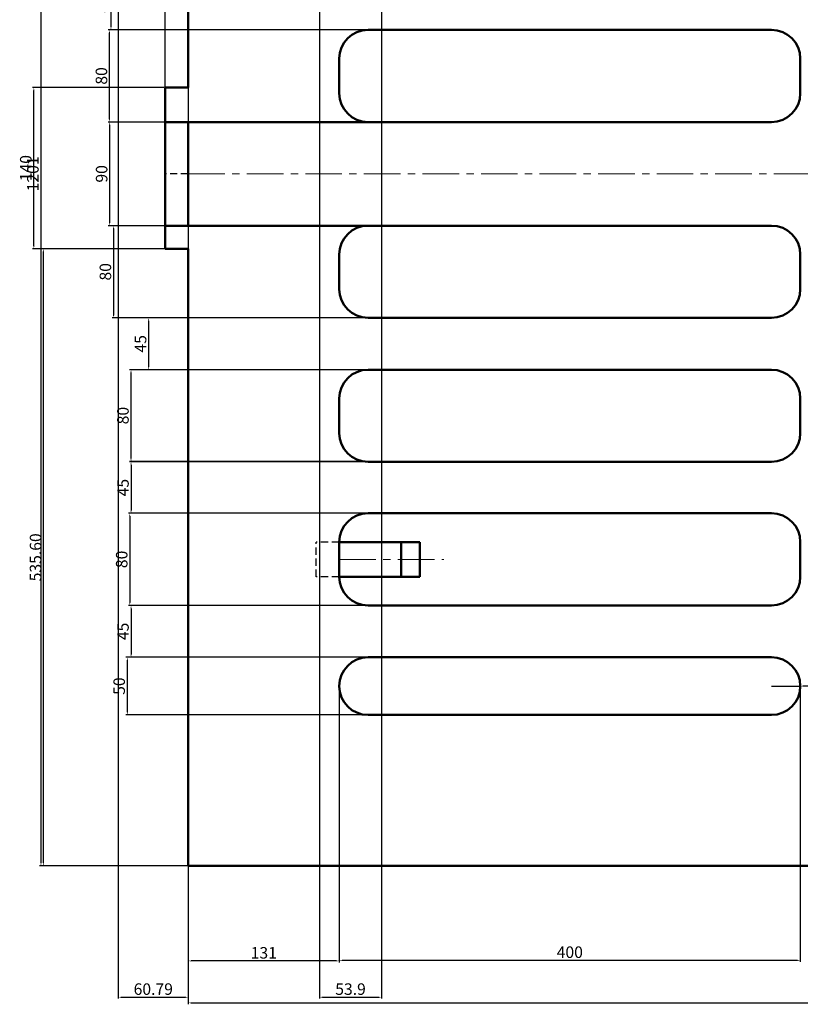
# Model space of a CAD drawing. Units: millimetres. Extents: x 1178 to 3717, y 924 to 2764.
# Tile 2 of 5: x 1793 to 2471, y 931 to 1785. Entities that reach past the tile are written whole.
import ezdxf

# ---------------------------------------------------------------- set-up
doc = ezdxf.new("R2010")
doc.units = ezdxf.units.MM
doc.linetypes.add('CENTER', pattern=[50.8, 31.75, -6.35, 6.35, -6.35])
doc.linetypes.add('HIDDEN', pattern=[9.525, 6.35, -3.175])
for name, color, linetype, lineweight in [('M-CNTR', 1, 'CENTER', 18), ('M-DIMS', 2, 'Continuous', 25), ('M-HIDN', 6, 'HIDDEN', 25), ('M-OUTL', 7, 'Continuous', 50)]:
    doc.layers.add(name, color=color, linetype=linetype, lineweight=lineweight)
doc.styles.get("Standard").update_dxf_attribs({"font": 'arial.ttf'})
doc.dimstyles.new('ISO-25', dxfattribs={"dimtxt": 10, "dimasz": 2.5, "dimexe": 1.25, "dimexo": 0.625, "dimtad": 1, "dimtoh": 1, "dimdec": 0, "dimtxsty": 'Standard', "dimcen": 2.5, "dimadec": 0, "dimazin": 0, "dimtfac": 1, "dimtdec": 0, "dimtmove": 0, "dimatfit": 3, "dimfxl": 1, "dimarcsym": 0})

# ---------------------------------------------------------------- blocks, each defined once
blk = doc.blocks.new('*D1')
at = {"layer": 'Defpoints', "color": 0, "transparency": 16777216}
for p in [(1939.54, 1051.02), (3521.54, 1051.02), (3521.54, 932.11)]:
    blk.add_point(p, dxfattribs=at)
at = {"layer": 'M-DIMS', "color": 0, "lineweight": -2, "transparency": 16777216}
for p, q in [((1939.54, 1050.4), (1939.54, 930.86)), ((3521.54, 1050.4), (3521.54, 930.86)), ((1942.04, 932.11), (3519.04, 932.11))]:
    blk.add_line(p, q, dxfattribs=at)
at = {"layer": 'M-DIMS', "color": 0, "transparency": 16777216}
for points in [[(1942.04, 932.53), (1942.04, 931.7), (1939.54, 932.11)], [(3519.04, 932.53), (3519.04, 931.7), (3521.54, 932.11)]]:
    blk.add_solid(points, dxfattribs=at)
at = {"layer": 'M-DIMS', "color": 0, "transparency": 16777216, "insert": (2730.54, 937.85), "char_height": 10, "attachment_point": 5}
blk.add_mtext('1582', dxfattribs=at)
blk = doc.blocks.new('*D2')
at = {"layer": 'Defpoints', "color": 0, "transparency": 16777216}
for p in [(1939.54, 2252.21), (1811.7, 1051.02), (1939.54, 1051.02)]:
    blk.add_point(p, dxfattribs=at)
at = {"layer": 'M-DIMS', "color": 0, "lineweight": -2, "transparency": 16777216}
for p, q in [((1938.91, 2252.21), (1810.45, 2252.21)), ((1811.7, 2249.71), (1811.7, 1053.52)), ((1938.91, 1051.02), (1810.45, 1051.02))]:
    blk.add_line(p, q, dxfattribs=at)
at = {"layer": 'M-DIMS', "color": 0, "transparency": 16777216}
for points in [[(1811.29, 2249.71), (1812.12, 2249.71), (1811.7, 2252.21)], [(1811.29, 1053.52), (1812.12, 1053.52), (1811.7, 1051.02)]]:
    blk.add_solid(points, dxfattribs=at)
at = {"layer": 'M-DIMS', "color": 0, "transparency": 16777216, "insert": (1805.97, 1651.62), "char_height": 10, "attachment_point": 5, "rotation": 90}
blk.add_mtext('1201', dxfattribs=at)
blk = doc.blocks.new('*D3')
at = {"layer": 'Defpoints', "color": 0, "transparency": 16777216}
for p in [(2070.54, 1207.02), (2470.54, 1207.02), (2470.54, 969.06)]:
    blk.add_point(p, dxfattribs=at)
at = {"layer": 'M-DIMS', "color": 0, "lineweight": -2, "transparency": 16777216}
for p, q in [((2070.54, 1206.4), (2070.54, 967.81)), ((2470.54, 1206.4), (2470.54, 967.81)), ((2073.04, 969.06), (2468.04, 969.06))]:
    blk.add_line(p, q, dxfattribs=at)
at = {"layer": 'M-DIMS', "color": 0, "transparency": 16777216}
for points in [[(2073.04, 969.48), (2073.04, 968.64), (2070.54, 969.06)], [(2468.04, 969.48), (2468.04, 968.64), (2470.54, 969.06)]]:
    blk.add_solid(points, dxfattribs=at)
at = {"layer": 'M-DIMS', "color": 0, "transparency": 16777216, "insert": (2270.54, 974.79), "char_height": 10, "attachment_point": 5}
blk.add_mtext('400', dxfattribs=at)
blk = doc.blocks.new('*D6')
at = {"layer": 'Defpoints', "color": 0, "transparency": 16777216}
for p in [(2095.54, 1232.02), (1886.58, 1182.02), (2095.54, 1182.02)]:
    blk.add_point(p, dxfattribs=at)
at = {"layer": 'M-DIMS', "color": 0, "lineweight": -2, "transparency": 16777216}
for p, q in [((2094.91, 1232.02), (1885.33, 1232.02)), ((1886.58, 1229.52), (1886.58, 1184.52)), ((2094.91, 1182.02), (1885.33, 1182.02))]:
    blk.add_line(p, q, dxfattribs=at)
at = {"layer": 'M-DIMS', "color": 0, "transparency": 16777216}
for points in [[(1886.16, 1229.52), (1886.99, 1229.52), (1886.58, 1232.02)], [(1886.16, 1184.52), (1886.99, 1184.52), (1886.58, 1182.02)]]:
    blk.add_solid(points, dxfattribs=at)
at = {"layer": 'M-DIMS', "color": 0, "transparency": 16777216, "insert": (1880.85, 1207.02), "char_height": 10, "attachment_point": 5, "rotation": 90}
blk.add_mtext('50', dxfattribs=at)
blk = doc.blocks.new('*D7')
at = {"layer": 'Defpoints', "color": 0, "transparency": 16777216}
for p in [(2095.54, 1277.02), (1889.85, 1232.02), (2095.54, 1232.02)]:
    blk.add_point(p, dxfattribs=at)
at = {"layer": 'M-DIMS', "color": 0, "lineweight": -2, "transparency": 16777216}
for p, q in [((2094.91, 1277.02), (1888.6, 1277.02)), ((1889.85, 1274.52), (1889.85, 1234.52)), ((2094.91, 1232.02), (1888.6, 1232.02))]:
    blk.add_line(p, q, dxfattribs=at)
at = {"layer": 'M-DIMS', "color": 0, "transparency": 16777216}
for points in [[(1889.43, 1274.52), (1890.27, 1274.52), (1889.85, 1277.02)], [(1889.43, 1234.52), (1890.27, 1234.52), (1889.85, 1232.02)]]:
    blk.add_solid(points, dxfattribs=at)
at = {"layer": 'M-DIMS', "color": 0, "transparency": 16777216, "insert": (1884.14, 1254.52), "char_height": 10, "attachment_point": 5, "rotation": 90}
blk.add_mtext('45', dxfattribs=at)
blk = doc.blocks.new('*D8')
at = {"layer": 'Defpoints', "color": 0, "transparency": 16777216}
for p in [(2095.54, 1357.02), (1888.76, 1277.02), (2095.54, 1277.02)]:
    blk.add_point(p, dxfattribs=at)
at = {"layer": 'M-DIMS', "color": 0, "lineweight": -2, "transparency": 16777216}
for p, q in [((2094.91, 1357.02), (1887.51, 1357.02)), ((1888.76, 1354.52), (1888.76, 1279.52)), ((2094.91, 1277.02), (1887.51, 1277.02))]:
    blk.add_line(p, q, dxfattribs=at)
at = {"layer": 'M-DIMS', "color": 0, "transparency": 16777216}
for points in [[(1888.34, 1354.52), (1889.18, 1354.52), (1888.76, 1357.02)], [(1888.34, 1279.52), (1889.18, 1279.52), (1888.76, 1277.02)]]:
    blk.add_solid(points, dxfattribs=at)
at = {"layer": 'M-DIMS', "color": 0, "transparency": 16777216, "insert": (1883.03, 1317.02), "char_height": 10, "attachment_point": 5, "rotation": 90}
blk.add_mtext('80', dxfattribs=at)
blk = doc.blocks.new('*D9')
at = {"layer": 'Defpoints', "color": 0, "transparency": 16777216}
for p in [(2095.54, 1401.62), (1889.85, 1357.02), (2095.54, 1357.02)]:
    blk.add_point(p, dxfattribs=at)
at = {"layer": 'M-DIMS', "color": 0, "lineweight": -2, "transparency": 16777216}
for p, q in [((2094.91, 1401.62), (1888.6, 1401.62)), ((1889.85, 1399.12), (1889.85, 1359.52)), ((2094.91, 1357.02), (1888.6, 1357.02))]:
    blk.add_line(p, q, dxfattribs=at)
at = {"layer": 'M-DIMS', "color": 0, "transparency": 16777216}
for points in [[(1889.43, 1399.12), (1890.27, 1399.12), (1889.85, 1401.62)], [(1889.43, 1359.52), (1890.27, 1359.52), (1889.85, 1357.02)]]:
    blk.add_solid(points, dxfattribs=at)
at = {"layer": 'M-DIMS', "color": 0, "transparency": 16777216, "insert": (1884.14, 1379.32), "char_height": 10, "attachment_point": 5, "rotation": 90}
blk.add_mtext('45', dxfattribs=at)
blk = doc.blocks.new('*D10')
at = {"layer": 'Defpoints', "color": 0, "transparency": 16777216}
for p in [(2095.54, 1526.62), (1905.12, 1481.62), (2095.54, 1481.62)]:
    blk.add_point(p, dxfattribs=at)
at = {"layer": 'M-DIMS', "color": 0, "lineweight": -2, "transparency": 16777216}
for p, q in [((2094.91, 1526.62), (1903.87, 1526.62)), ((1905.12, 1524.12), (1905.12, 1484.12)), ((2094.91, 1481.62), (1903.87, 1481.62))]:
    blk.add_line(p, q, dxfattribs=at)
at = {"layer": 'M-DIMS', "color": 0, "transparency": 16777216}
for points in [[(1904.71, 1524.12), (1905.54, 1524.12), (1905.12, 1526.62)], [(1904.71, 1484.12), (1905.54, 1484.12), (1905.12, 1481.62)]]:
    blk.add_solid(points, dxfattribs=at)
at = {"layer": 'M-DIMS', "color": 0, "transparency": 16777216, "insert": (1899.41, 1504.12), "char_height": 10, "attachment_point": 5, "rotation": 90}
blk.add_mtext('45', dxfattribs=at)
blk = doc.blocks.new('*D11')
at = {"layer": 'Defpoints', "color": 0, "transparency": 16777216}
for p in [(1889.85, 1481.62), (2095.54, 1481.62), (2095.54, 1402.02)]:
    blk.add_point(p, dxfattribs=at)
at = {"layer": 'M-DIMS', "color": 0, "lineweight": -2, "transparency": 16777216}
for p, q in [((2094.91, 1481.62), (1888.6, 1481.62)), ((1889.85, 1404.52), (1889.85, 1479.12)), ((2094.91, 1402.02), (1888.6, 1402.02))]:
    blk.add_line(p, q, dxfattribs=at)
at = {"layer": 'M-DIMS', "color": 0, "transparency": 16777216}
for points in [[(1889.43, 1479.12), (1890.27, 1479.12), (1889.85, 1481.62)], [(1889.43, 1404.52), (1890.27, 1404.52), (1889.85, 1402.02)]]:
    blk.add_solid(points, dxfattribs=at)
at = {"layer": 'M-DIMS', "color": 0, "transparency": 16777216, "insert": (1884.12, 1441.82), "char_height": 10, "attachment_point": 5, "rotation": 90}
blk.add_mtext('80', dxfattribs=at)
blk = doc.blocks.new('*D12')
at = {"layer": 'Defpoints', "color": 0, "transparency": 16777216}
for p in [(2095.54, 1606.62), (1874.63, 1526.62), (2095.54, 1526.62)]:
    blk.add_point(p, dxfattribs=at)
at = {"layer": 'M-DIMS', "color": 0, "lineweight": -2, "transparency": 16777216}
for p, q in [((2094.91, 1606.62), (1873.38, 1606.62)), ((1874.63, 1604.12), (1874.63, 1529.12)), ((2094.91, 1526.62), (1873.38, 1526.62))]:
    blk.add_line(p, q, dxfattribs=at)
at = {"layer": 'M-DIMS', "color": 0, "transparency": 16777216}
for points in [[(1874.22, 1604.12), (1875.05, 1604.12), (1874.63, 1606.62)], [(1874.22, 1529.12), (1875.05, 1529.12), (1874.63, 1526.62)]]:
    blk.add_solid(points, dxfattribs=at)
at = {"layer": 'M-DIMS', "color": 0, "transparency": 16777216, "insert": (1868.9, 1566.62), "char_height": 10, "attachment_point": 5, "rotation": 90}
blk.add_mtext('80', dxfattribs=at)
blk = doc.blocks.new('*D13')
at = {"layer": 'Defpoints', "color": 0, "transparency": 16777216}
for p in [(1871.36, 1696.62), (2095.54, 1696.62), (2095.54, 1606.62)]:
    blk.add_point(p, dxfattribs=at)
at = {"layer": 'M-DIMS', "color": 0, "lineweight": -2, "transparency": 16777216}
for p, q in [((2094.91, 1696.62), (1870.11, 1696.62)), ((1871.36, 1609.12), (1871.36, 1694.12)), ((2094.91, 1606.62), (1870.11, 1606.62))]:
    blk.add_line(p, q, dxfattribs=at)
at = {"layer": 'M-DIMS', "color": 0, "transparency": 16777216}
for points in [[(1870.94, 1694.12), (1871.78, 1694.12), (1871.36, 1696.62)], [(1870.94, 1609.12), (1871.78, 1609.12), (1871.36, 1606.62)]]:
    blk.add_solid(points, dxfattribs=at)
at = {"layer": 'M-DIMS', "color": 0, "transparency": 16777216, "insert": (1865.63, 1651.62), "char_height": 10, "attachment_point": 5, "rotation": 90}
blk.add_mtext('90', dxfattribs=at)
blk = doc.blocks.new('*D14')
at = {"layer": 'Defpoints', "color": 0, "transparency": 16777216}
for p in [(2095.54, 1821.62), (1872.45, 1776.62), (2095.54, 1776.62)]:
    blk.add_point(p, dxfattribs=at)
at = {"layer": 'M-DIMS', "color": 0, "lineweight": -2, "transparency": 16777216}
for p, q in [((2094.91, 1821.62), (1871.2, 1821.62)), ((1872.45, 1819.12), (1872.45, 1779.12)), ((2094.91, 1776.62), (1871.2, 1776.62))]:
    blk.add_line(p, q, dxfattribs=at)
at = {"layer": 'M-DIMS', "color": 0, "transparency": 16777216}
for points in [[(1872.03, 1819.12), (1872.87, 1819.12), (1872.45, 1821.62)], [(1872.03, 1779.12), (1872.87, 1779.12), (1872.45, 1776.62)]]:
    blk.add_solid(points, dxfattribs=at)
at = {"layer": 'M-DIMS', "color": 0, "transparency": 16777216, "insert": (1866.74, 1799.12), "char_height": 10, "attachment_point": 5, "rotation": 90}
blk.add_mtext('45', dxfattribs=at)
blk = doc.blocks.new('*D15')
at = {"layer": 'Defpoints', "color": 0, "transparency": 16777216}
for p in [(1871.2, 1776.62), (2095.54, 1776.62), (2095.54, 1696.62)]:
    blk.add_point(p, dxfattribs=at)
at = {"layer": 'M-DIMS', "color": 0, "lineweight": -2, "transparency": 16777216}
for p, q in [((2094.91, 1776.62), (1869.95, 1776.62)), ((1871.2, 1699.12), (1871.2, 1774.12)), ((2094.91, 1696.62), (1869.95, 1696.62))]:
    blk.add_line(p, q, dxfattribs=at)
at = {"layer": 'M-DIMS', "color": 0, "transparency": 16777216}
for points in [[(1870.78, 1774.12), (1871.62, 1774.12), (1871.2, 1776.62)], [(1870.78, 1699.12), (1871.62, 1699.12), (1871.2, 1696.62)]]:
    blk.add_solid(points, dxfattribs=at)
at = {"layer": 'M-DIMS', "color": 0, "transparency": 16777216, "insert": (1865.47, 1736.62), "char_height": 10, "attachment_point": 5, "rotation": 90}
blk.add_mtext('80', dxfattribs=at)
blk = doc.blocks.new('*D21')
at = {"layer": 'Defpoints', "color": 0, "transparency": 16777216}
for p in [(1939.54, 1318.82), (2070.54, 1207.02), (1939.54, 968.52)]:
    blk.add_point(p, dxfattribs=at)
at = {"layer": 'M-DIMS', "color": 0, "lineweight": -2, "transparency": 16777216}
for p, q in [((1939.54, 1318.2), (1939.54, 967.27)), ((2070.54, 1206.4), (2070.54, 967.27)), ((2068.04, 968.52), (1942.04, 968.52))]:
    blk.add_line(p, q, dxfattribs=at)
at = {"layer": 'M-DIMS', "color": 0, "transparency": 16777216}
for points in [[(1942.04, 968.93), (1942.04, 968.1), (1939.54, 968.52)], [(2068.04, 968.93), (2068.04, 968.1), (2070.54, 968.52)]]:
    blk.add_solid(points, dxfattribs=at)
at = {"layer": 'M-DIMS', "color": 0, "transparency": 16777216, "insert": (2005.04, 974.25), "char_height": 10, "attachment_point": 5}
blk.add_mtext('131', dxfattribs=at)
blk = doc.blocks.new('SLOT-400X50')
for p, q in [((375, 50), (25, 50)), ((25, 0), (375, 0))]:
    blk.add_line(p, q)
for centre, start, end in [((25, 25), 90, 270), ((375, 25), 270, 90)]:
    blk.add_arc(centre, 25, start, end)
blk = doc.blocks.new('*D28')
at = {"layer": 'Defpoints', "color": 0, "transparency": 16777216}
for p in [(1878.75, 2626.04), (1939.54, 2504.04), (1939.54, 937.02)]:
    blk.add_point(p, dxfattribs=at)
at = {"layer": 'M-DIMS', "color": 0, "lineweight": -2, "transparency": 16777216}
for p, q in [((1878.75, 2625.42), (1878.75, 935.77)), ((1939.54, 2503.42), (1939.54, 935.77)), ((1881.25, 937.02), (1937.04, 937.02))]:
    blk.add_line(p, q, dxfattribs=at)
at = {"layer": 'M-DIMS', "color": 0, "transparency": 16777216}
for points in [[(1881.25, 937.44), (1881.25, 936.61), (1878.75, 937.02)], [(1937.04, 937.44), (1937.04, 936.61), (1939.54, 937.02)]]:
    blk.add_solid(points, dxfattribs=at)
at = {"layer": 'M-DIMS', "color": 0, "transparency": 16777216, "insert": (1909.15, 942.75), "char_height": 10, "attachment_point": 5}
blk.add_mtext('60.79', dxfattribs=at)
blk = doc.blocks.new('*D43')
at = {"layer": 'Defpoints', "color": 0, "transparency": 16777216}
for p in [(2053.34, 2567.8), (2107.24, 2567.8), (2107.24, 937.02)]:
    blk.add_point(p, dxfattribs=at)
at = {"layer": 'M-DIMS', "color": 0, "lineweight": -2, "transparency": 16777216}
for p, q in [((2053.34, 2567.18), (2053.34, 935.77)), ((2107.24, 2567.18), (2107.24, 935.77)), ((2055.84, 937.02), (2104.74, 937.02))]:
    blk.add_line(p, q, dxfattribs=at)
at = {"layer": 'M-DIMS', "color": 0, "transparency": 16777216}
for points in [[(2055.84, 937.44), (2055.84, 936.61), (2053.34, 937.02)], [(2104.74, 937.44), (2104.74, 936.61), (2107.24, 937.02)]]:
    blk.add_solid(points, dxfattribs=at)
at = {"layer": 'M-DIMS', "color": 0, "transparency": 16777216, "insert": (2080.29, 942.76), "char_height": 10, "attachment_point": 5}
blk.add_mtext('53.9', dxfattribs=at)
blk = doc.blocks.new('*D55')
at = {"layer": 'Defpoints', "color": 0, "transparency": 16777216}
for p in [(1939.54, 1840.62), (1919.54, 1726.62), (1939.54, 1726.62)]:
    blk.add_point(p, dxfattribs=at)
at = {"layer": 'M-DIMS', "color": 0, "lineweight": -2, "transparency": 16777216}
for p, q in [((1919.54, 1727.24), (1919.54, 1841.87)), ((1922.04, 1840.62), (1937.04, 1840.62)), ((1939.54, 1727.24), (1939.54, 1841.87))]:
    blk.add_line(p, q, dxfattribs=at)
at = {"layer": 'M-DIMS', "color": 0, "transparency": 16777216}
for points in [[(1922.04, 1841.03), (1922.04, 1840.2), (1919.54, 1840.62)], [(1937.04, 1841.03), (1937.04, 1840.2), (1939.54, 1840.62)]]:
    blk.add_solid(points, dxfattribs=at)
at = {"layer": 'M-DIMS', "color": 0, "transparency": 16777216, "insert": (1929.54, 1846.35), "char_height": 10, "attachment_point": 5}
blk.add_mtext('20', dxfattribs=at)
blk = doc.blocks.new('*D56')
at = {"layer": 'Defpoints', "color": 0, "transparency": 16777216}
for p in [(1805.54, 1726.62), (1919.54, 1726.62), (1919.54, 1586.62)]:
    blk.add_point(p, dxfattribs=at)
at = {"layer": 'M-DIMS', "color": 0, "lineweight": -2, "transparency": 16777216}
for p, q in [((1918.91, 1726.62), (1804.29, 1726.62)), ((1805.54, 1589.12), (1805.54, 1724.12)), ((1918.91, 1586.62), (1804.29, 1586.62))]:
    blk.add_line(p, q, dxfattribs=at)
at = {"layer": 'M-DIMS', "color": 0, "transparency": 16777216}
for points in [[(1805.12, 1724.12), (1805.96, 1724.12), (1805.54, 1726.62)], [(1805.12, 1589.12), (1805.96, 1589.12), (1805.54, 1586.62)]]:
    blk.add_solid(points, dxfattribs=at)
at = {"layer": 'M-DIMS', "color": 0, "transparency": 16777216, "insert": (1799.81, 1656.62), "char_height": 10, "attachment_point": 5, "rotation": 90}
blk.add_mtext('140', dxfattribs=at)
blk = doc.blocks.new('*D70')
at = {"layer": 'Defpoints', "color": 0, "transparency": 16777216}
for p in [(1814.04, 1586.62), (1939.54, 1586.62), (1939.54, 1051.02)]:
    blk.add_point(p, dxfattribs=at)
at = {"layer": 'M-DIMS', "color": 0, "lineweight": -2, "transparency": 16777216}
for p, q in [((1938.91, 1586.62), (1812.79, 1586.62)), ((1814.04, 1053.52), (1814.04, 1584.12)), ((1938.91, 1051.02), (1812.79, 1051.02))]:
    blk.add_line(p, q, dxfattribs=at)
at = {"layer": 'M-DIMS', "color": 0, "transparency": 16777216}
for points in [[(1813.62, 1584.12), (1814.46, 1584.12), (1814.04, 1586.62)], [(1813.62, 1053.52), (1814.46, 1053.52), (1814.04, 1051.02)]]:
    blk.add_solid(points, dxfattribs=at)
at = {"layer": 'M-DIMS', "color": 0, "transparency": 16777216, "insert": (1808.31, 1318.82), "char_height": 10, "attachment_point": 5, "rotation": 90}
blk.add_mtext('535.60', dxfattribs=at)
blk = doc.blocks.new('*D99')
at = {"layer": 'Defpoints', "color": 0, "transparency": 16777216}
for p in [(2445.54, 1207.02), (2470.54, 1207.02)]:
    blk.add_point(p, dxfattribs=at)
at = {"layer": 'M-DIMS', "color": 0, "lineweight": -2, "transparency": 16777216}
for p, q in [((2445.54, 1207.02), (2470.54, 1207.02)), ((2485.75, 1207.02), (2473.04, 1207.02)), ((2529.66, 1207.02), (2485.75, 1207.02))]:
    blk.add_line(p, q, dxfattribs=at)
at = {"layer": 'M-DIMS', "color": 0, "transparency": 16777216}
blk.add_solid([(2473.04, 1207.44), (2473.04, 1206.6), (2470.54, 1207.02)], dxfattribs=at)
at = {"layer": 'M-DIMS', "color": 0, "transparency": 16777216, "insert": (2508.02, 1212.75), "char_height": 10, "attachment_point": 5}
blk.add_mtext('R25.00', dxfattribs=at)

msp = doc.modelspace()

# ---------------------------------------------------------------- linework, layer by layer
at = {"layer": 'M-CNTR'}
for p, q in [((1939.5398, 1651.6179), (3521.5398, 1651.6179)), ((2070.5398, 1317.0224), (2161.1852, 1317.0224))]:
    msp.add_line(p, q, dxfattribs=at)
at = {"layer": 'M-HIDN'}
for p, q in [((1939.5398, 1651.6179), (1919.5398, 1651.6179)), ((1939.5398, 1606.6179), (1939.5398, 1651.6179)), ((2070.5398, 1332.0224), (2050.6046, 1332.0224)), ((2050.6046, 1302.0224), (2050.6046, 1332.0224)), ((2070.5398, 1302.0224), (2050.6046, 1302.0224))]:
    msp.add_line(p, q, dxfattribs=at)
at = {"layer": 'M-OUTL'}
for p, q in [((1939.5398, 1903.0224), (1939.5398, 1726.6179)), ((2095.5398, 1776.6179), (2445.5398, 1776.6179)), ((2070.5398, 1751.6179), (2070.5398, 1721.6179)), ((2470.5398, 1751.6179), (2470.5398, 1721.6179)), ((1919.5398, 1586.6179), (1919.5398, 1726.6179)), ((1919.5398, 1726.6179), (1939.5398, 1726.6179)), ((1939.5398, 1696.6179), (1919.5398, 1696.6179)), ((2095.5398, 1696.6179), (1939.5398, 1696.6179)), ((1939.5398, 1696.6179), (1939.5398, 1606.6179)), ((2445.5398, 1696.6179), (2095.5398, 1696.6179)), ((1939.5398, 1606.6179), (1919.5398, 1606.6179)), ((2095.5398, 1606.6179), (1939.5398, 1606.6179)), ((2445.5398, 1606.6179), (2095.5398, 1606.6179)), ((1939.5398, 1586.6179), (1919.5398, 1586.6179)), ((1939.5398, 1586.6179), (1939.5398, 1051.0224)), ((2070.5398, 1551.6179), (2070.5398, 1581.6179)), ((2470.5398, 1551.6179), (2470.5398, 1581.6179)), ((2095.5398, 1526.6179), (2445.5398, 1526.6179)), ((2445.5398, 1481.6179), (2095.5398, 1481.6179)), ((2070.5398, 1456.6179), (2070.5398, 1426.6179)), ((2470.5398, 1426.6179), (2470.5398, 1456.6179)), ((2095.5398, 1401.6179), (2095.5398, 1402.0224)), ((2095.5398, 1401.6179), (2445.5398, 1401.6179)), ((2445.5398, 1357.0224), (2095.5398, 1357.0224)), ((2070.5398, 1332.0224), (2070.5398, 1302.0224)), ((2070.5398, 1332.0224), (2140.3627, 1332.0224)), ((2124.325, 1332.0224), (2124.325, 1302.0224)), ((2140.3627, 1302.0224), (2140.3627, 1332.0224)), ((2470.5398, 1302.0224), (2470.5398, 1332.0224)), ((2070.5398, 1302.0224), (2140.3627, 1302.0224)), ((2095.5398, 1277.0224), (2445.5398, 1277.0224)), ((1939.5398, 1051.0224), (3521.5398, 1051.0224)), ((1939.5398, 1051.0224), (2070.5398, 1051.0224))]:
    msp.add_line(p, q, dxfattribs=at)
for centre, start, end in [((2095.5398, 1751.6179), 90, 180), ((2445.5398, 1751.6179), 0, 90), ((2095.5398, 1721.6179), 180, 270), ((2445.5398, 1721.6179), 270, 0), ((2095.5398, 1581.6179), 90, 180), ((2445.5398, 1581.6179), 0, 90), ((2095.5398, 1551.6179), 180, 270), ((2445.5398, 1551.6179), 270, 0), ((2095.5398, 1456.6179), 90, 180), ((2445.5398, 1456.6179), 0, 90), ((2095.5398, 1426.6179), 180, 270), ((2445.5398, 1426.6179), 270, 0), ((2095.5398, 1332.0224), 90, 180), ((2445.5398, 1332.0224), 0, 90), ((2095.5398, 1302.0224), 180, 270), ((2445.5398, 1302.0224), 270, 0)]:
    msp.add_arc(centre, 25, start, end, dxfattribs=at)

# ---------------------------------------------------------------- block references
msp.add_blockref('SLOT-400X50', (2070.54, 1182.022), dxfattribs=at)

# ---------------------------------------------------------------- dimensions: what is measured, and where the dimension line sits
at = {"layer": 'M-DIMS'}
for base, p1, p2, override, picture, middle in [((1939.5398, 937.0224), (1878.7536, 2626.0416), (1939.5398, 2504.0416), {"dimdec": 2, "dimlfac": 1, "dimrnd": 0, "dimzin": 0, "dimdsep": 46, "dimlunit": 2}, '*D28', (1909.1467, 942.7532)), ((2107.2394, 937.0224), (2053.3369, 2567.8003), (2107.2394, 2567.8003), {"dimdec": 1, "dimlfac": 1, "dimrnd": 0, "dimzin": 0, "dimdsep": 46, "dimlunit": 2}, '*D43', (2080.2882, 942.7566)), ((1939.5398, 1840.6179), (1919.5398, 1726.6179), (1939.5398, 1726.6179), {"dimdec": 0, "dimlfac": 1, "dimrnd": 0, "dimzin": 0, "dimdsep": 46, "dimlunit": 2}, '*D55', (1929.5398, 1846.3487)), ((1939.5398, 968.5153), (2070.5398, 1207.0224), (1939.5398, 1318.8202), {"dimclrd": 0, "dimclre": 0, "dimclrt": 0}, '*D21', (2005.0398, 974.2494)), ((2470.5398, 969.0589), (2070.5398, 1207.0224), (2470.5398, 1207.0224), {"dimclrd": 0, "dimclre": 0, "dimclrt": 0}, '*D3', (2270.5398, 974.7897)), ((3521.5398, 932.1144), (1939.5398, 1051.0224), (3521.5398, 1051.0224), {"dimclrd": 0, "dimclre": 0, "dimclrt": 0}, '*D1', (2730.5398, 937.8451))]:
    dim = msp.add_linear_dim(base=base, p1=p1, p2=p2, dimstyle='ISO-25', override=override, dxfattribs=at)
    dim.commit()
    dim.dimension.update_dxf_attribs({"geometry": picture, "text_midpoint": middle})
for base, p1, p2, override, picture, middle in [((1811.7032, 1051.0224), (1939.5398, 2252.2134), (1939.5398, 1051.0224), {"dimclrd": 0, "dimclre": 0, "dimclrt": 0}, '*D2', (1805.9725, 1651.6179)), ((1872.4506, 1776.6179), (2095.5398, 1821.6179), (2095.5398, 1776.6179), {"dimclrd": 0, "dimclre": 0, "dimclrt": 0}, '*D14', (1866.7404, 1799.1179)), ((1871.2006, 1776.6179), (2095.5398, 1696.6179), (2095.5398, 1776.6179), {"dimclrd": 0, "dimclre": 0, "dimclrt": 0}, '*D15', (1865.4699, 1736.6179)), ((1805.5398, 1726.6179), (1919.5398, 1586.6179), (1919.5398, 1726.6179), {"dimdec": 0, "dimlfac": 1, "dimrnd": 0, "dimzin": 0, "dimdsep": 46, "dimlunit": 2}, '*D56', (1799.8091, 1656.6179)), ((1871.3596, 1696.6179), (2095.5398, 1606.6179), (2095.5398, 1696.6179), {"dimclrd": 0, "dimclre": 0, "dimclrt": 0}, '*D13', (1865.6289, 1651.6179)), ((1874.6326, 1526.6179), (2095.5398, 1606.6179), (2095.5398, 1526.6179), {"dimclrd": 0, "dimclre": 0, "dimclrt": 0}, '*D12', (1868.9019, 1566.6179)), ((1814.0398, 1586.6179), (1939.5398, 1051.0224), (1939.5398, 1586.6179), {"dimdec": 2, "dimlfac": 1, "dimrnd": 0, "dimzin": 0, "dimdsep": 46, "dimlunit": 2}, '*D70', (1808.3057, 1318.8202)), ((1905.1249, 1481.6179), (2095.5398, 1526.6179), (2095.5398, 1481.6179), {"dimclrd": 0, "dimclre": 0, "dimclrt": 0}, '*D10', (1899.4146, 1504.1179)), ((1889.851, 1481.6179), (2095.5398, 1402.0224), (2095.5398, 1481.6179), {"dimclrd": 0, "dimclre": 0, "dimclrt": 0}, '*D11', (1884.1203, 1441.8202)), ((1889.851, 1357.0224), (2095.5398, 1401.6179), (2095.5398, 1357.0224), {"dimclrd": 0, "dimclre": 0, "dimclrt": 0}, '*D9', (1884.1408, 1379.3202)), ((1888.76, 1277.0224), (2095.5398, 1357.0224), (2095.5398, 1277.0224), {"dimclrd": 0, "dimclre": 0, "dimclrt": 0}, '*D8', (1883.0293, 1317.0224)), ((1889.851, 1232.0224), (2095.5398, 1277.0224), (2095.5398, 1232.0224), {"dimclrd": 0, "dimclre": 0, "dimclrt": 0}, '*D7', (1884.1408, 1254.5224)), ((1886.578, 1182.0224), (2095.5398, 1232.0224), (2095.5398, 1182.0224), {"dimclrd": 0, "dimclre": 0, "dimclrt": 0}, '*D6', (1880.8473, 1207.0224))]:
    dim = msp.add_linear_dim(base=base, p1=p1, p2=p2, angle=90, dimstyle='ISO-25', override=override, dxfattribs=at)
    dim.commit()
    dim.dimension.update_dxf_attribs({"geometry": picture, "text_midpoint": middle})
dim = msp.add_radius_dim(center=(2445.5398, 1207.0224), mpoint=(2470.5398, 1207.02), dimstyle='ISO-25', override={"dimdec": 2, "dimlfac": 1, "dimrnd": 0, "dimzin": 0, "dimdsep": 46, "dimlunit": 2}, dxfattribs=at)
dim.commit()
dim.dimension.update_dxf_attribs({"geometry": '*D99', "text_midpoint": (2508.0168, 1212.7492)})

doc.saveas('drawing.dxf')
